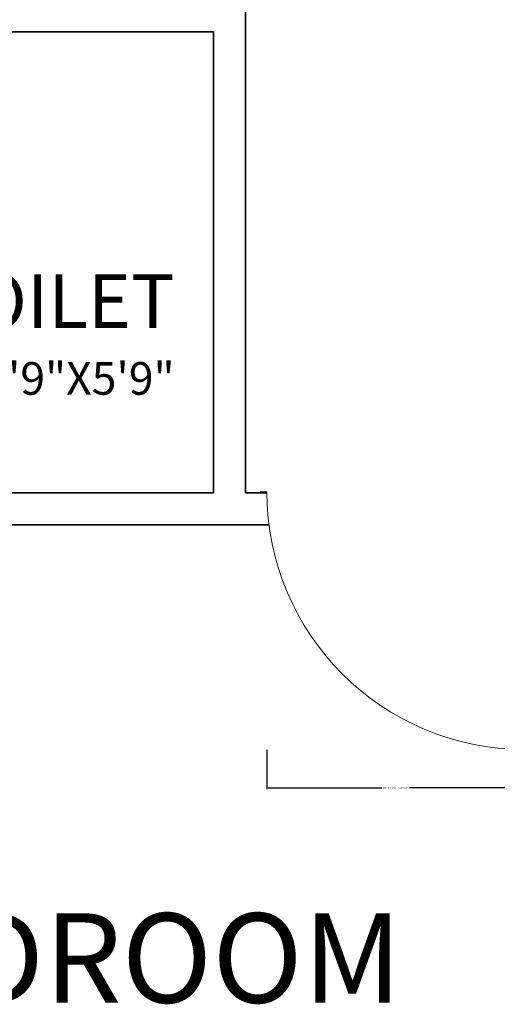
# Model space of a CAD drawing. Units: inches. Extents: x -26 to 788, y -42 to 505.
# Tile 3 of 9: x 49 to 116, y 124 to 262. Entities that reach past the tile are written whole.
import ezdxf

# ---------------------------------------------------------------- set-up
doc = ezdxf.new("R2010")
doc.units = ezdxf.units.IN
doc.header["$MEASUREMENT"] = 0
for name, color, linetype, lineweight in [('A-ANNO-DIMS', 2, 'Continuous', 18), ('A-AREA-IDEN', 7, 'Continuous', 18), ('A-DOOR', 3, 'Continuous', 18), ('A-WALL', 7, 'Continuous', 35)]:
    doc.layers.add(name, color=color, linetype=linetype, lineweight=lineweight)
doc.styles.get("Standard").update_dxf_attribs({"font": 'arial.ttf'})
doc.dimstyles.get("Standard").update_dxf_attribs({"dimtxt": 0.18, "dimasz": 0.18, "dimexe": 0.18, "dimexo": 0.0625, "dimgap": 0.09, "dimtad": 0, "dimtih": 1, "dimtoh": 1, "dimdec": 4, "dimzin": 0, "dimdsep": 46, "dimtxsty": 'Standard', "dimcen": 0.09, "dimadec": 0, "dimazin": 0, "dimtfac": 1, "dimtdec": 4, "dimtofl": 0, "dimtmove": 0, "dimatfit": 3, "dimfxl": 1, "dimtolj": 1, "dimtzin": 0, "dimarcsym": 0})

# ---------------------------------------------------------------- blocks, each defined once
blk = doc.blocks.new('DOOR-BEDROOM-36')
blk.add_line((36, 0), (36, 36))
blk.add_arc((36, 36), 36, 180, 270)
blk = doc.blocks.new('*D35')
at = {"layer": 'A-ANNO-DIMS', "color": 0, "lineweight": -2, "transparency": 16777216}
for p, q in [((83.95, 159.65), (83.95, 154.13)), ((119.95, 159.65), (119.95, 154.13)), ((84.13, 154.31), (100.02, 154.31)), ((119.77, 154.31), (103.89, 154.31))]:
    blk.add_line(p, q, dxfattribs=at)
at = {"layer": 'A-ANNO-DIMS', "color": 0, "transparency": 16777216}
for points in [[(84.13, 154.34), (84.13, 154.28), (83.95, 154.31)], [(119.77, 154.34), (119.77, 154.28), (119.95, 154.31)]]:
    blk.add_solid(points, dxfattribs=at)
at = {"layer": 'Defpoints', "color": 0, "transparency": 16777216}
for p in [(83.95, 159.71), (119.95, 159.71), (119.95, 154.31)]:
    blk.add_point(p, dxfattribs=at)
at = {"layer": 'A-ANNO-DIMS', "color": 0, "transparency": 16777216, "insert": (101.95, 154.31), "char_height": 0.18, "attachment_point": 5}
blk.add_mtext('\\A1;BEDROOM DOOR 36.0000 TYP.', dxfattribs=at)

msp = doc.modelspace()

# ---------------------------------------------------------------- linework, layer by layer
at = {"layer": 'A-WALL'}
for p, q in [((80.95497, 195.61777), (80.95497, 283.96697)), ((11.95497, 260.11777), (76.45497, 260.11777)), ((76.45497, 195.61777), (76.45497, 260.11777)), ((38.88227, 195.61777), (76.45497, 195.61777)), ((80.95497, 195.61777), (83.95508, 195.61777)), ((83.95497, 195.70898), (82.99754, 195.70898)), ((39.17022, 191.11777), (84.24893, 191.11777))]:
    msp.add_line(p, q, dxfattribs=at)

# ---------------------------------------------------------------- block references
at = {"layer": 'A-DOOR'}
msp.add_blockref('DOOR-BEDROOM-36', (83.955, 159.709), dxfattribs=at)

# ---------------------------------------------------------------- texts
at = {"layer": 'A-AREA-IDEN'}
for s, height, p in [('TOILET', 7.483862, (36.68656, 218.68186)), ('5\'9"X5\'9"', 4.56659, (44.26822, 209.32026)), ('BEDROOM', 12.516013, (19.77046, 124.25891))]:
    msp.add_text(s, height=height, dxfattribs=at).set_placement(p)

# ---------------------------------------------------------------- dimensions: what is measured, and where the dimension line sits
at = {"layer": 'A-ANNO-DIMS'}
dim = msp.add_linear_dim(base=(119.95497, 154.30898), p1=(83.95497, 159.70898), p2=(119.95497, 159.70898), text='BEDROOM DOOR <> TYP.', dimstyle='Standard', override={"dimdec": 4, "dimlfac": 1, "dimrnd": 0, "dimzin": 0, "dimdsep": 46, "dimlunit": 2}, dxfattribs=at)
dim.commit()
dim.dimension.update_dxf_attribs({"geometry": '*D35', "text_midpoint": (101.95497, 154.30898)})

doc.saveas('drawing.dxf')
